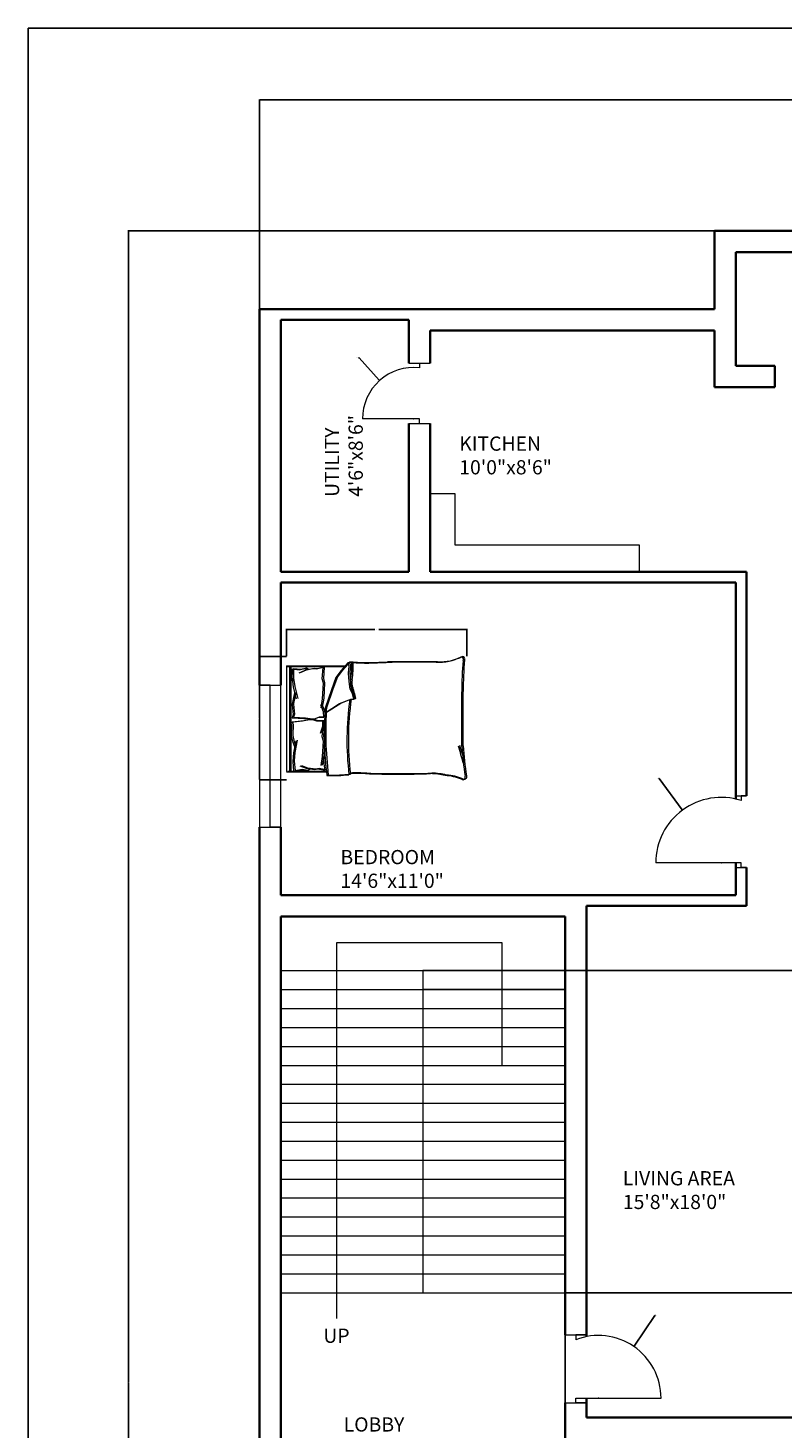
# Model space of a CAD drawing. Units: inches. Extents: x 1902 to 2626, y 1199 to 2408.
# Tile 6 of 9: x 1902 to 2220, y 1817 to 2408. Entities that reach past the tile are written whole.
import ezdxf

# ---------------------------------------------------------------- set-up
doc = ezdxf.new("R2010")
doc.units = ezdxf.units.IN
for name, color, linetype, lineweight in [('A-ANNO-DIMS', 2, 'Continuous', 18), ('A-ANNO-SYMB', 52, 'Continuous', 13), ('A-ANNO-TTLB', 7, 'Continuous', 25), ('A-AREA-IDEN', 7, 'Continuous', 18), ('A-DOOR', 31, 'Continuous', 18), ('A-FLOR-CASE', 8, 'Continuous', 18), ('A-FLOR-STRS', 52, 'Continuous', 18), ('A-FURN', 8, 'Continuous', 13), ('A-GLAZ', 181, 'Continuous', 18), ('A-WALL', 7, 'Continuous', 35)]:
    doc.layers.add(name, color=color, linetype=linetype, lineweight=lineweight)
doc.styles.get("Standard").update_dxf_attribs({"font": 'arial.ttf'})
doc.dimstyles.get("Standard").update_dxf_attribs({"dimtxt": 0.18, "dimasz": 0.18, "dimexe": 0.18, "dimexo": 0.0625, "dimgap": 0.09, "dimtad": 0, "dimtih": 1, "dimtoh": 1, "dimdec": 4, "dimzin": 0, "dimdsep": 46, "dimtxsty": 'Standard', "dimcen": 0.09, "dimadec": 0, "dimazin": 0, "dimtfac": 1, "dimtdec": 4, "dimtofl": 0, "dimtmove": 0, "dimatfit": 3, "dimfxl": 1, "dimtolj": 1, "dimtzin": 0, "dimarcsym": 0})

# ---------------------------------------------------------------- blocks, each defined once
blk = doc.blocks.new('BED-DOUBLE')
for p, q in [((-0.01, 48.09), (0.59, 48.09)), ((-0.01, 48.09), (-0.01, 3.46)), ((-0.01, 47.87), (24.84, 47.87)), ((-0.01, 47.87), (24.84, 47.87)), ((0.59, 48.09), (25.44, 48.09)), ((0.59, 48.09), (25.44, 48.09)), ((1.43, 3.25), (1.43, 47.87)), ((1.43, 3.25), (1.43, 47.87)), ((2.02, 3.46), (2.02, 48.09)), ((2.02, 3.46), (2.02, 48.09)), ((15.47, 47.34), (12.54, 46.62)), ((15.47, 47.34), (12.54, 46.62)), ((16.07, 47.56), (13.14, 46.83)), ((16.07, 47.56), (13.14, 46.83)), ((15.09, 42.55), (15.47, 47.34)), ((15.09, 42.55), (15.47, 47.34)), ((15.69, 42.77), (16.07, 47.56)), ((15.69, 42.77), (16.07, 47.56)), ((25.9, 49.37), (22.87, 45.91)), ((25.9, 49.37), (22.87, 45.91)), ((26.5, 49.58), (23.46, 46.12)), ((26.5, 49.58), (23.46, 46.12)), ((27.53, 49.44), (25.9, 49.37, 3.61)), ((27.53, 49.44), (25.9, 49.37, 3.61)), ((26.48, 47.93), (25.9, 49.37)), ((26.48, 47.93), (25.9, 49.37)), ((26.19, 45.04), (26.48, 47.93)), ((26.19, 45.04), (26.48, 47.93)), ((28.13, 49.66), (26.5, 49.58, 3.61)), ((28.13, 49.66), (26.5, 49.58, 3.61)), ((27.08, 48.15), (26.5, 49.58)), ((27.08, 48.15), (26.5, 49.58)), ((26.79, 45.26), (27.08, 48.15)), ((26.79, 45.25), (27.08, 48.15)), ((2.38, 46.8), (2.29, 41.75)), ((2.38, 46.8), (2.29, 41.75)), ((2.29, 41.75), (2.37, 42.69)), ((2.29, 41.75), (2.37, 42.69)), ((2.37, 42.69), (2.86, 39.14)), ((2.37, 42.69), (2.86, 39.14)), ((2.38, 46.8), (5.38, 46.44)), ((2.38, 46.8), (5.38, 46.44)), ((2.98, 47.01), (2.89, 41.97)), ((2.98, 47.01), (2.89, 41.96)), ((2.89, 41.97), (2.97, 42.9)), ((2.89, 41.96), (2.97, 42.9)), ((2.97, 42.9), (3.46, 39.36)), ((2.97, 42.9), (3.46, 39.35)), ((2.98, 47.01), (5.98, 46.66)), ((2.98, 47.01), (5.98, 46.66)), ((7.7, 46.05), (5.2, 44.94)), ((7.7, 46.05), (5.2, 44.94)), ((5.38, 46.44), (7.78, 47)), ((5.38, 46.44), (7.78, 47)), ((8.3, 46.26), (5.8, 45.16)), ((8.3, 46.26), (5.8, 45.16)), ((5.98, 46.66), (8.38, 47.21)), ((5.98, 46.66), (8.38, 47.21)), ((11.04, 46.8), (7.7, 46.05)), ((11.04, 46.8), (7.7, 46.05)), ((7.78, 47), (8.76, 46.52)), ((7.78, 47), (8.76, 46.52)), ((11.64, 47.01), (8.3, 46.26)), ((11.64, 47.01), (8.3, 46.26)), ((8.38, 47.21), (9.35, 46.73)), ((8.38, 47.21), (9.35, 46.73)), ((12.54, 46.62), (11.04, 46.8)), ((12.54, 46.62), (11.04, 46.8)), ((13.14, 46.83), (11.64, 47.01)), ((13.14, 46.83), (11.64, 47.01)), ((15.61, 40.72), (15.09, 42.55)), ((15.61, 40.72), (15.09, 42.55)), ((16.21, 40.93), (15.69, 42.77)), ((16.21, 40.93), (15.69, 42.77)), ((20.84, 43.16), (18.97, 37.96)), ((20.84, 43.16), (18.97, 37.96)), ((21.44, 43.38), (19.56, 38.17)), ((21.44, 43.38), (19.56, 38.17)), ((22.87, 45.91), (20.84, 43.16)), ((22.87, 45.91), (20.84, 43.16)), ((23.46, 46.12), (21.44, 43.38)), ((23.46, 46.12), (21.44, 43.38)), ((26.48, 41.43), (26.19, 45.04)), ((26.48, 41.43), (26.19, 45.04)), ((26.91, 38.25), (26.48, 41.43)), ((26.91, 38.24), (26.48, 41.43)), ((27.08, 41.64), (26.79, 45.26)), ((27.08, 41.64), (26.79, 45.25)), ((27.51, 38.46), (27.08, 41.64)), ((27.51, 38.46), (27.08, 41.64)), ((2.86, 39.14), (4.12, 34.08)), ((2.86, 39.14), (4.12, 34.08)), ((3.42, 36.61), (2.87, 34.68)), ((3.42, 36.61), (2.87, 34.68)), ((3.46, 39.36), (4.72, 34.29)), ((3.46, 39.35), (4.72, 34.29)), ((4.02, 36.82), (3.47, 34.89)), ((4.02, 36.82), (3.47, 34.89)), ((15.21, 34.18), (15.61, 40.72)), ((15.21, 34.18), (15.61, 40.72)), ((15.81, 34.39), (16.21, 40.93)), ((15.81, 34.39), (16.21, 40.93)), ((18.97, 37.96), (16.23, 30.17)), ((18.97, 37.96), (16.23, 30.17)), ((19.56, 38.17), (16.82, 30.38)), ((19.56, 38.17), (16.82, 30.38)), ((27.78, 36.37), (26.91, 38.25)), ((27.78, 36.36), (26.91, 38.24)), ((28.38, 36.58), (27.51, 38.46)), ((28.38, 36.58), (27.51, 38.46)), ((28.36, 34.05), (27.78, 36.37)), ((28.36, 34.05), (27.78, 36.36)), ((28.96, 34.26), (28.38, 36.58)), ((28.96, 34.26), (28.38, 36.58)), ((73.99, 14.07), (73.99, 37.05)), ((73.99, 14.07), (73.99, 37.05)), ((74.59, 14.28), (74.59, 37.27)), ((74.59, 14.28), (74.59, 37.27)), ((2.87, 34.68), (2.36, 31.94)), ((2.87, 34.68), (2.36, 31.94)), ((2.36, 31.94), (2.38, 31.64)), ((2.36, 31.94), (2.38, 31.64)), ((2.38, 31.64), (2.78, 27.51)), ((2.38, 31.64), (2.78, 27.51)), ((3.47, 34.89), (2.96, 32.16)), ((3.47, 34.89), (2.96, 32.16)), ((2.96, 32.16), (2.98, 31.86)), ((2.96, 32.16), (2.98, 31.86)), ((2.98, 31.86), (3.37, 27.72)), ((2.98, 31.86), (3.37, 27.72)), ((15.63, 28.72), (14.43, 31.58)), ((15.63, 28.72), (14.43, 31.58)), ((14.59, 30.41), (15.21, 34.18)), ((14.59, 30.41), (15.21, 34.18)), ((16.22, 28.93), (15.02, 31.8)), ((16.22, 28.93), (15.02, 31.8)), ((15.18, 30.62), (15.81, 34.39)), ((15.18, 30.62), (15.81, 34.39)), ((16.23, 28.26), (22.29, 32.17)), ((16.23, 28.26), (22.29, 32.17)), ((16.82, 28.47), (22.89, 32.38)), ((16.82, 28.47), (22.89, 32.38)), ((22.29, 32.17), (26.48, 33.76)), ((22.29, 32.17), (26.48, 33.76)), ((22.89, 32.38), (27.08, 33.98)), ((22.89, 32.38), (27.08, 33.98)), ((26.48, 33.76), (28.36, 34.05)), ((26.48, 33.76), (28.36, 34.05)), ((27.08, 33.98), (28.96, 34.26)), ((27.08, 33.98), (28.96, 34.26)), ((1.74, 24.27), (6.74, 24.81)), ((1.74, 24.27), (6.74, 24.81)), ((2.28, 22.92), (1.74, 24.27)), ((2.28, 22.92), (1.74, 24.27)), ((2.78, 27.51), (2.32, 26.13)), ((2.78, 27.51), (2.32, 26.13)), ((2.32, 26.13), (7.34, 25.9)), ((2.32, 26.13), (7.34, 25.9)), ((2.34, 24.48), (7.33, 25.02)), ((2.34, 24.48), (7.33, 25.02)), ((2.88, 23.13), (2.34, 24.48)), ((2.88, 23.13), (2.34, 24.48)), ((3.37, 27.72), (2.92, 26.34)), ((3.37, 27.72), (2.92, 26.34)), ((2.92, 26.34), (7.94, 26.11)), ((2.92, 26.34), (7.94, 26.11)), ((6.74, 24.81), (9.71, 25.35)), ((6.74, 24.81), (9.71, 25.35)), ((7.33, 25.02), (10.3, 25.56)), ((7.33, 25.02), (10.3, 25.56)), ((7.34, 25.9), (10.34, 25.55)), ((7.34, 25.9), (10.34, 25.55)), ((7.94, 26.11), (10.94, 25.76)), ((7.94, 26.11), (10.94, 25.76)), ((9.71, 25.35), (10.92, 25.35)), ((9.71, 25.35), (10.92, 25.35)), ((10.3, 25.56), (11.52, 25.56)), ((10.3, 25.56), (11.52, 25.56)), ((10.34, 25.55), (11.55, 25.62)), ((10.34, 25.55), (11.55, 25.62)), ((10.92, 25.35), (12.68, 24.81)), ((10.92, 25.35), (12.68, 24.81)), ((10.94, 25.76), (12.15, 25.84)), ((10.94, 25.76), (12.15, 25.84)), ((11.52, 25.56), (13.27, 25.02)), ((11.52, 25.56), (13.27, 25.02)), ((11.55, 25.62), (13.27, 26.27)), ((11.55, 25.62), (13.27, 26.27)), ((12.15, 25.84), (13.87, 26.48)), ((12.15, 25.84), (13.87, 26.48)), ((12.68, 24.81), (15.18, 24.81)), ((12.68, 24.81), (15.18, 24.81)), ((13.27, 26.27), (15.77, 26.43)), ((13.27, 26.27), (15.77, 26.43)), ((13.27, 25.02), (15.78, 25.02)), ((13.27, 25.02), (15.78, 25.02)), ((13.87, 26.48), (16.37, 26.64)), ((13.87, 26.48), (16.37, 26.64)), ((15.18, 24.81), (15.18, 22.51)), ((15.18, 24.81), (15.18, 22.51)), ((15.77, 26.43), (15.63, 28.72)), ((15.77, 26.43), (15.63, 28.72)), ((15.78, 25.02), (15.78, 22.72)), ((15.78, 25.02), (15.78, 22.72)), ((16.37, 26.64), (16.22, 28.93)), ((16.37, 26.64), (16.22, 28.93)), ((2.15, 18.76), (2.28, 22.92)), ((2.15, 18.76), (2.28, 22.92)), ((2.15, 18.46), (2.15, 18.76)), ((2.15, 18.46), (2.15, 18.76)), ((2.82, 15.76), (2.15, 18.46)), ((2.82, 15.76), (2.15, 18.46)), ((2.74, 18.98), (2.88, 23.13)), ((2.74, 18.98), (2.88, 23.13)), ((2.74, 18.68), (2.74, 18.98)), ((2.74, 18.68), (2.74, 18.98)), ((3.42, 15.98), (2.74, 18.68)), ((3.42, 15.98), (2.74, 18.68)), ((15.18, 22.51), (14.16, 19.57)), ((15.18, 22.51), (14.16, 19.57)), ((15.78, 22.72), (14.76, 19.79)), ((15.78, 22.72), (14.76, 19.79)), ((15.09, 18.1), (15.47, 22.9)), ((15.09, 18.1), (15.47, 22.9)), ((15.61, 16.27), (15.09, 18.1)), ((15.61, 16.27), (15.09, 18.1)), ((15.69, 18.32), (16.07, 23.11)), ((15.69, 18.32), (16.07, 23.11)), ((16.21, 16.49), (15.69, 18.32)), ((16.21, 16.49), (15.69, 18.32)), ((3.5, 13.88), (2.82, 15.76)), ((3.5, 13.87), (2.82, 15.76)), ((3.09, 11.31), (4.04, 16.44)), ((3.09, 11.31), (4.04, 16.44)), ((4.09, 14.09), (3.42, 15.98)), ((4.09, 14.09), (3.42, 15.98)), ((3.69, 11.52), (4.63, 16.65)), ((3.69, 11.52), (4.63, 16.65)), ((15.21, 9.73), (15.61, 16.27)), ((15.21, 9.73), (15.61, 16.27)), ((15.81, 9.94), (16.21, 16.49)), ((15.81, 9.94), (16.21, 16.49)), ((2.8, 7.64), (2.82, 7.74)), ((2.8, 7.64), (2.82, 7.74)), ((3.11, 3.64), (2.8, 7.64)), ((3.11, 3.64), (2.8, 7.64)), ((2.82, 7.74), (3.09, 11.31)), ((2.82, 7.74), (3.09, 11.31)), ((3.4, 7.86), (3.42, 7.95)), ((3.4, 7.86), (3.42, 7.95)), ((3.71, 3.86), (3.4, 7.86)), ((3.71, 3.86), (3.4, 7.86)), ((3.42, 7.95), (3.69, 11.52)), ((3.42, 7.95), (3.69, 11.52)), ((14.59, 5.96), (15.21, 9.73)), ((14.59, 5.96), (15.21, 9.73)), ((15.18, 6.18), (15.81, 9.94)), ((15.18, 6.18), (15.81, 9.94)), ((15.21, 9.73), (15.51, 8.67)), ((15.21, 9.73), (15.51, 8.67)), ((15.51, 8.67), (16.19, 3.91)), ((15.51, 8.67), (16.19, 3.91)), ((15.81, 9.94), (16.11, 8.88)), ((15.81, 9.94), (16.11, 8.88)), ((16.11, 8.88), (16.78, 4.12)), ((16.11, 8.88), (16.78, 4.12)), ((16.91, 3.25), (-0.01, 3.25)), ((16.91, 3.25), (-0.01, 3.25)), ((17.5, 3.46), (0.59, 3.46)), ((17.5, 3.46), (0.59, 3.46)), ((3.09, 3.64), (6.06, 4.18)), ((3.09, 3.64), (6.06, 4.18)), ((3.69, 3.85), (6.66, 4.39)), ((3.69, 3.85), (6.66, 4.39)), ((8.36, 4.72), (5.79, 5.67)), ((8.36, 4.72), (5.79, 5.67)), ((6.06, 4.18), (8.49, 3.78)), ((6.06, 4.18), (8.49, 3.78)), ((8.95, 4.93), (6.39, 5.88)), ((8.95, 4.93), (6.39, 5.88)), ((6.66, 4.39), (9.09, 3.99)), ((6.66, 4.39), (9.09, 3.99)), ((11.73, 4.18), (8.36, 4.72)), ((11.73, 4.18), (8.36, 4.72)), ((8.49, 3.78), (9.44, 4.32)), ((8.49, 3.78), (9.44, 4.32)), ((12.33, 4.39), (8.95, 4.93)), ((12.33, 4.39), (8.95, 4.93)), ((9.09, 3.99), (10.03, 4.53)), ((9.09, 3.99), (10.03, 4.53)), ((13.22, 4.45), (11.73, 4.18)), ((13.22, 4.45), (11.73, 4.18)), ((13.81, 4.66), (12.33, 4.39)), ((13.81, 4.66), (12.33, 4.39)), ((16.19, 3.91), (13.22, 4.45)), ((16.19, 3.91), (13.22, 4.45)), ((16.78, 4.12), (13.81, 4.66)), ((16.78, 4.12), (13.81, 4.66))]:
    blk.add_line(p, q)
for centre, radius, start, end in [((-6.22, 47.93), 33.79, 349.87628, 2.56571), ((-6.22, 47.93), 33.79, 349.87628, 2.56571), ((33.9, 170.19), 120.92, 266.97912, 273.83645), ((33.9, 170.19), 120.92, 266.97912, 273.83645), ((-5.62, 48.14), 33.79, 349.87628, 2.56571), ((-5.62, 48.14), 33.79, 349.87628, 2.56571), ((34.5, 170.41), 120.92, 266.97912, 273.83645), ((34.5, 170.41), 120.92, 266.97912, 273.83645), ((63.32, -4210.02), 4259.62, 90.00217, 90.28689), ((63.32, -4210.02), 4259.62, 90.00217, 90.28689), ((63.92, -4209.8), 4259.62, 90.00217, 90.28689), ((63.92, -4209.8), 4259.62, 90.00217, 90.28689), ((64.11, 71.12), 21.54, 267.47136, 296.46809), ((64.11, 71.12), 21.54, 267.47136, 296.46809), ((64.71, 71.33), 21.54, 267.47136, 296.46809), ((64.71, 71.33), 21.54, 267.47136, 296.46809), ((73.64, 50.81), 1.03, 332.65876, 86.02002), ((73.64, 50.81), 1.03, 332.65876, 86.02002), ((198.21, 38.43), 124.23, 174.4998, 180.63509), ((198.21, 38.43), 124.23, 174.4998, 180.63509), ((74.24, 51.02), 1.03, 332.65876, 86.02002), ((74.24, 51.02), 1.03, 332.65876, 86.02002), ((198.8, 38.64), 124.23, 174.4998, 180.63509), ((198.8, 38.64), 124.23, 174.4998, 180.63509), ((32.74, 40.85), 5.81, 168.6608, 203.73842), ((32.74, 40.85), 5.81, 168.6608, 203.73842), ((33.33, 41.06), 5.81, 168.6608, 203.73842), ((33.33, 41.06), 5.81, 168.6608, 203.73842), ((1.38, 29.09), 27.69, 10.66171, 19.88058), ((1.38, 29.09), 27.69, 10.66171, 19.88058), ((1.98, 29.31), 27.69, 10.66171, 19.88058), ((1.98, 29.31), 27.69, 10.66171, 19.88058), ((169.99, 19.95), 154.04, 176.08655, 186.78213), ((169.99, 19.95), 154.04, 176.08655, 186.78213), ((170.58, 20.16), 154.04, 176.08655, 186.78213), ((170.58, 20.16), 154.04, 176.08655, 186.78213), ((145.95, 16.58), 120.47, 171.78449, 186.90062), ((145.95, 16.58), 120.47, 171.78449, 186.90062), ((146.55, 16.8), 120.47, 171.78449, 186.90062), ((146.55, 16.8), 120.47, 171.78449, 186.90062), ((28.42, 34.21), 0.172, 250.24637, 1.13765), ((28.42, 34.21), 0.172, 250.24637, 1.13765), ((29.01, 34.43), 0.172, 250.24637, 1.13765), ((29.01, 34.43), 0.172, 250.24637, 1.13765), ((-22.15, -16.08), 99.41, 13.38322, 17.70533), ((-22.15, -16.08), 99.41, 13.38322, 17.70533), ((-21.55, -15.86), 99.41, 13.38322, 17.70533), ((-21.55, -15.86), 99.41, 13.38322, 17.70533), ((187.53, 20.01), 113.69, 182.99578, 189.40907), ((187.53, 20.01), 113.69, 182.99578, 189.40907), ((188.12, 20.22), 113.69, 182.99578, 189.40907), ((188.12, 20.22), 113.69, 182.99578, 189.40907), ((18.76, 79.52), 77.79, 268.72178, 275.60397), ((18.76, 79.52), 77.79, 268.72178, 275.60397), ((19.36, 79.74), 77.79, 268.72178, 275.60397), ((19.36, 79.74), 77.79, 268.72178, 275.60397), ((29.1, -156.22), 158.84, 88.4762, 91.00819), ((29.1, -156.22), 158.84, 88.4762, 91.00819), ((29.7, -156), 158.84, 88.4762, 91.00819), ((29.7, -156.01), 158.84, 88.4762, 91.00819), ((47.26, 452.71), 450.36, 268.22771, 271.71854), ((47.26, 452.71), 450.36, 268.22771, 271.71854), ((47.85, 452.92), 450.36, 268.22771, 271.71854), ((47.85, 452.92), 450.36, 268.22771, 271.71854), ((60.24, -25.11), 27.67, 76.06484, 88.91125), ((60.24, -25.11), 27.67, 76.06484, 88.91125), ((60.83, -24.9), 27.67, 76.06484, 88.91125), ((60.83, -24.9), 27.67, 76.06484, 88.91125), ((65.61, -20.22), 22, 67.97508, 86.652), ((65.61, -20.22), 22, 67.97508, 86.652), ((66.21, -20.01), 22, 67.97508, 86.652), ((66.21, -20.01), 22, 67.97508, 86.652), ((74.43, 1.02), 1.02, 236.17358, 23.47814), ((74.43, 1.02), 1.02, 236.17358, 23.47814), ((75.03, 1.23), 1.02, 236.17358, 23.47814), ((75.03, 1.23), 1.02, 236.17358, 23.47814)]:
    blk.add_arc(centre, radius, start, end)
blk = doc.blocks.new('WINDOW-60-A')
for p, q in [((0, 9), (0, 0)), ((60, 9), (0, 9)), ((60, 4.5), (60, 9)), ((60, 9), (60, 0)), ((0, 0), (0, 4.5)), ((0, 4.5), (60, 4.5)), ((0, 0), (60, 0))]:
    blk.add_line(p, q)
blk = doc.blocks.new('*D10')
at = {"layer": 'A-ANNO-DIMS', "color": 0, "lineweight": -2, "transparency": 16777216}
for p, q in [((2010.79, 2142.84), (2010.79, 2154.38)), ((2010.97, 2154.2), (2048.05, 2154.2)), ((2086.76, 2154.2), (2049.69, 2154.2)), ((2086.94, 2142.84), (2086.94, 2154.38))]:
    blk.add_line(p, q, dxfattribs=at)
at = {"layer": 'A-ANNO-DIMS', "color": 0, "transparency": 16777216}
for points in [[(2010.97, 2154.23), (2010.97, 2154.17), (2010.79, 2154.2)], [(2086.76, 2154.23), (2086.76, 2154.17), (2086.94, 2154.2)]]:
    blk.add_solid(points, dxfattribs=at)
at = {"layer": 'Defpoints', "color": 0, "transparency": 16777216}
for p in [(2086.94, 2154.2), (2010.79, 2142.78), (2086.94, 2142.78)]:
    blk.add_point(p, dxfattribs=at)
at = {"layer": 'A-ANNO-DIMS', "color": 0, "transparency": 16777216, "insert": (2048.87, 2154.2), "char_height": 0.18, "attachment_point": 5}
blk.add_mtext('\\A1;BED 76 TYP.', dxfattribs=at)
blk = doc.blocks.new('*D11')
at = {"layer": 'A-ANNO-DIMS', "color": 0, "lineweight": -2, "transparency": 16777216}
for p, q in [((2010.73, 2142.78), (1999.19, 2142.78)), ((1999.37, 2142.6), (1999.37, 2116.9)), ((1999.37, 2090.83), (1999.37, 2116.53)), ((2010.73, 2090.65), (1999.19, 2090.65))]:
    blk.add_line(p, q, dxfattribs=at)
at = {"layer": 'A-ANNO-DIMS', "color": 0, "transparency": 16777216}
for points in [[(1999.34, 2142.6), (1999.4, 2142.6), (1999.37, 2142.78)], [(1999.34, 2090.83), (1999.4, 2090.83), (1999.37, 2090.65)]]:
    blk.add_solid(points, dxfattribs=at)
at = {"layer": 'Defpoints', "color": 0, "transparency": 16777216}
for p in [(1999.37, 2142.78), (2010.79, 2142.78), (2010.79, 2090.65)]:
    blk.add_point(p, dxfattribs=at)
at = {"layer": 'A-ANNO-DIMS', "color": 0, "transparency": 16777216, "insert": (1999.37, 2116.72), "char_height": 0.18, "attachment_point": 5}
blk.add_mtext('\\A1;52 TYP.', dxfattribs=at)
blk = doc.blocks.new('*D28')
at = {"layer": 'A-ANNO-DIMS', "color": 0, "lineweight": -2, "transparency": 16777216}
for p, q in [((1999.35, 2289.54), (1999.35, 2377.95)), ((1999.53, 2377.77), (2268.21, 2377.77)), ((2537.67, 2377.77), (2269, 2377.77)), ((2537.85, 2289.54), (2537.85, 2377.95))]:
    blk.add_line(p, q, dxfattribs=at)
at = {"layer": 'A-ANNO-DIMS', "color": 0, "transparency": 16777216}
for points in [[(1999.53, 2377.8), (1999.53, 2377.74), (1999.35, 2377.77)], [(2537.67, 2377.8), (2537.67, 2377.74), (2537.85, 2377.77)]]:
    blk.add_solid(points, dxfattribs=at)
at = {"layer": 'Defpoints', "color": 0, "transparency": 16777216}
for p in [(2537.85, 2377.77), (1999.35, 2289.47), (2537.85, 2289.47)]:
    blk.add_point(p, dxfattribs=at)
at = {"layer": 'A-ANNO-DIMS', "color": 0, "transparency": 16777216, "insert": (2268.6, 2377.77), "char_height": 0.18, "attachment_point": 5}
blk.add_mtext('\\A1;538.5', dxfattribs=at)
blk = doc.blocks.new('*D29')
at = {"layer": 'A-ANNO-DIMS', "color": 0, "lineweight": -2, "transparency": 16777216}
for p, q in [((2191.29, 2322.47), (1943.87, 2322.47)), ((1944.05, 2322.29), (1944.05, 1836.38)), ((1944.05, 1350.11), (1944.05, 1836.02)), ((2202.79, 1349.93), (1943.87, 1349.93))]:
    blk.add_line(p, q, dxfattribs=at)
at = {"layer": 'A-ANNO-DIMS', "color": 0, "transparency": 16777216}
for points in [[(1944.02, 2322.29), (1944.08, 2322.29), (1944.05, 2322.47)], [(1944.02, 1350.11), (1944.08, 1350.11), (1944.05, 1349.93)]]:
    blk.add_solid(points, dxfattribs=at)
at = {"layer": 'Defpoints', "color": 0, "transparency": 16777216}
for p in [(1944.05, 2322.47), (2191.35, 2322.47), (2202.85, 1349.93)]:
    blk.add_point(p, dxfattribs=at)
at = {"layer": 'A-ANNO-DIMS', "color": 0, "transparency": 16777216, "insert": (1944.05, 1836.2), "char_height": 0.18, "attachment_point": 5}
blk.add_mtext('\\A1;972.5', dxfattribs=at)
blk = doc.blocks.new('*D38')
at = {"layer": 'A-ANNO-DIMS', "color": 0, "lineweight": -2, "transparency": 16777216}
for p, q in [((2008.35, 1874.05), (2008.35, 1198.67)), ((2128.35, 1874.05), (2128.35, 1198.67)), ((2008.53, 1198.85), (2068.07, 1198.85)), ((2128.17, 1198.85), (2068.63, 1198.85))]:
    blk.add_line(p, q, dxfattribs=at)
at = {"layer": 'A-ANNO-DIMS', "color": 0, "transparency": 16777216}
for points in [[(2008.53, 1198.88), (2008.53, 1198.82), (2008.35, 1198.85)], [(2128.17, 1198.88), (2128.17, 1198.82), (2128.35, 1198.85)]]:
    blk.add_solid(points, dxfattribs=at)
at = {"layer": 'Defpoints', "color": 0, "transparency": 16777216}
for p in [(2008.35, 1874.11), (2128.35, 1874.11), (2128.35, 1198.85)]:
    blk.add_point(p, dxfattribs=at)
at = {"layer": 'A-ANNO-DIMS', "color": 0, "transparency": 16777216, "insert": (2068.35, 1198.85), "char_height": 0.18, "attachment_point": 5}
blk.add_mtext('\\A1;120', dxfattribs=at)
blk = doc.blocks.new('*D39')
at = {"layer": 'A-ANNO-DIMS', "color": 0, "lineweight": -2, "transparency": 16777216}
for p, q in [((2128.41, 2010.11), (2593.33, 2010.11)), ((2593.15, 2009.93), (2593.15, 1942.29)), ((2593.15, 1874.29), (2593.15, 1941.93)), ((2128.41, 1874.11), (2593.33, 1874.11))]:
    blk.add_line(p, q, dxfattribs=at)
at = {"layer": 'A-ANNO-DIMS', "color": 0, "transparency": 16777216}
for points in [[(2593.12, 2009.93), (2593.18, 2009.93), (2593.15, 2010.11)], [(2593.12, 1874.29), (2593.18, 1874.29), (2593.15, 1874.11)]]:
    blk.add_solid(points, dxfattribs=at)
at = {"layer": 'Defpoints', "color": 0, "transparency": 16777216}
for p in [(2128.35, 2010.11), (2593.15, 2010.11), (2128.35, 1874.11)]:
    blk.add_point(p, dxfattribs=at)
at = {"layer": 'A-ANNO-DIMS', "color": 0, "transparency": 16777216, "insert": (2593.15, 1942.11), "char_height": 0.18, "attachment_point": 5}
blk.add_mtext('\\A1;136', dxfattribs=at)
blk = doc.blocks.new('*D50')
at = {"layer": 'A-ANNO-DIMS', "color": 0, "lineweight": -2, "transparency": 16777216}
for p, q in [((2167.93, 2091.29), (2168.11, 2091.29)), ((2168.11, 2091.29), (2177.81, 2078.05)), ((2194.17, 2055.59), (2194.35, 2055.59)), ((2194.26, 2055.5), (2194.26, 2055.68))]:
    blk.add_line(p, q, dxfattribs=at)
at = {"layer": 'A-ANNO-DIMS', "color": 0, "transparency": 16777216}
blk.add_solid([(2177.83, 2078.07), (2177.78, 2078.03), (2177.92, 2077.9)], dxfattribs=at)
at = {"layer": 'Defpoints', "color": 0, "transparency": 16777216}
for p in [(2177.92, 2077.9), (2194.26, 2055.59)]:
    blk.add_point(p, dxfattribs=at)
at = {"layer": 'A-ANNO-DIMS', "color": 0, "transparency": 16777216, "insert": (2167.38, 2091.29), "char_height": 0.18, "attachment_point": 5}
blk.add_mtext('\\A1;R27.657', dxfattribs=at)
blk = doc.blocks.new('*D52')
at = {"layer": 'A-ANNO-DIMS', "color": 0, "lineweight": -2, "transparency": 16777216}
for p, q in [((2166.29, 1864.52), (2157.45, 1851.59)), ((2166.47, 1864.52), (2166.29, 1864.52)), ((2142.35, 1829.63), (2142.53, 1829.63)), ((2142.44, 1829.54), (2142.44, 1829.72))]:
    blk.add_line(p, q, dxfattribs=at)
at = {"layer": 'A-ANNO-DIMS', "color": 0, "transparency": 16777216}
blk.add_solid([(2157.42, 1851.6), (2157.47, 1851.57), (2157.34, 1851.44)], dxfattribs=at)
at = {"layer": 'Defpoints', "color": 0, "transparency": 16777216}
for p in [(2157.34, 1851.44), (2142.44, 1829.63)]:
    blk.add_point(p, dxfattribs=at)
at = {"layer": 'A-ANNO-DIMS', "color": 0, "transparency": 16777216, "insert": (2167.02, 1864.52), "char_height": 0.18, "attachment_point": 5}
blk.add_mtext('\\A1;R26.414', dxfattribs=at)
blk = doc.blocks.new('*D54')
at = {"layer": 'A-ANNO-DIMS', "color": 0, "lineweight": -2, "transparency": 16777216}
for p, q in [((2041.2, 2268.92), (2041.38, 2268.92)), ((2041.38, 2268.92), (2049.93, 2259.39)), ((2064.4, 2243.14), (2064.58, 2243.14)), ((2064.49, 2243.05), (2064.49, 2243.23))]:
    blk.add_line(p, q, dxfattribs=at)
at = {"layer": 'A-ANNO-DIMS', "color": 0, "transparency": 16777216}
blk.add_solid([(2049.95, 2259.41), (2049.91, 2259.37), (2050.05, 2259.25)], dxfattribs=at)
at = {"layer": 'Defpoints', "color": 0, "transparency": 16777216}
for p in [(2050.05, 2259.25), (2064.49, 2243.14)]:
    blk.add_point(p, dxfattribs=at)
at = {"layer": 'A-ANNO-DIMS', "color": 0, "transparency": 16777216, "insert": (2040.66, 2268.92), "char_height": 0.18, "attachment_point": 5}
blk.add_mtext('\\A1;R21.636', dxfattribs=at)

msp = doc.modelspace()

# ---------------------------------------------------------------- linework, layer by layer
at = {"layer": 'A-ANNO-SYMB'}
for p, q in [((2032.059, 1863.1842), (2032.059, 2022.0098)), ((2032.059, 2022.0098), (2101.6557, 2022.0098)), ((2101.6557, 2022.0098), (2101.6557, 1970.11)), ((2101.6557, 1970.11), (2101.6557, 1970.11))]:
    msp.add_line(p, q, dxfattribs=at)
at = {"layer": 'A-ANNO-TTLB'}
msp.add_lwpolyline([(1901.6928, 2408.1473), (2626.1646, 2408.1473), (2626.1646, 1206.3103), (1901.6928, 1206.3103)], close=True, dxfattribs=at)
at = {"layer": 'A-DOOR'}
for p, q in [((2062.3507, 2266.6459), (2071.3507, 2266.6459)), ((2066.8507, 2266.6459), (2066.8507, 2264.6459)), ((2066.8507, 2243.1399), (2042.8507, 2243.1399)), ((2062.3507, 2241.1399), (2071.3507, 2241.1399)), ((2066.8507, 2241.1399), (2066.8507, 2243.1399)), ((2200.3507, 2083.9588), (2204.8507, 2083.9588)), ((2204.8507, 2083.9588), (2202.6007, 2083.9588)), ((2202.6007, 2083.9588), (2202.6007, 2081.9588)), ((2202.6007, 2055.5908), (2166.6007, 2055.5908)), ((2200.3507, 2053.5908), (2204.8507, 2053.5908)), ((2202.6007, 2053.5908), (2202.6007, 2055.5908)), ((2204.8507, 2053.5908), (2202.6007, 2053.5908)), ((2128.3507, 1856.2475), (2137.3507, 1856.2475)), ((2137.3507, 1856.2475), (2132.8507, 1856.2475)), ((2132.8507, 1856.2475), (2132.8507, 1854.2475)), ((2128.3507, 1827.6338), (2137.3507, 1827.6338)), ((2132.8507, 1827.6338), (2132.8507, 1829.6338)), ((2132.8507, 1829.6338), (2168.8507, 1829.6338)), ((2137.3507, 1827.6338), (2132.8507, 1827.6338))]:
    msp.add_line(p, q, dxfattribs=at)
for centre, radius, start, end in [((2064.4863, 2243.1399), 21.6356, 83.7259546, 180), ((2194.2573, 2055.5908), 27.6566, 72.4414808, 180), ((2142.4363, 1829.6338), 26.4144, 0, 111.2780943)]:
    msp.add_arc(centre, radius, start, end, dxfattribs=at)
at = {"layer": 'A-FLOR-CASE'}
for p, q in [((2071.3507, 2211.5459), (2081.7541, 2211.5459)), ((2081.7541, 2211.5459), (2081.7541, 2189.8841)), ((2081.7541, 2189.8841), (2159.6685, 2189.8841)), ((2159.6685, 2189.8841), (2159.6685, 2178.4733))]:
    msp.add_line(p, q, dxfattribs=at)
at = {"layer": 'A-FLOR-STRS'}
for p, q in [((2008.3507, 2010.11), (2128.3507, 2010.11)), ((2128.3507, 2010.11), (2068.3507, 2010.11)), ((2068.3507, 2010.11), (2068.3507, 1874.11)), ((2008.3507, 2002.11), (2128.3507, 2002.11)), ((2128.3507, 2002.11), (2068.3507, 2002.11)), ((2008.3507, 1994.11), (2128.3507, 1994.11)), ((2008.3507, 1986.11), (2128.3507, 1986.11)), ((2008.3507, 1978.11), (2128.3507, 1978.11)), ((2008.3507, 1970.11), (2128.3507, 1970.11)), ((2008.3507, 1962.11), (2128.3507, 1962.11)), ((2008.3507, 1954.11), (2128.3507, 1954.11)), ((2008.3507, 1946.11), (2128.3507, 1946.11)), ((2008.3507, 1938.11), (2128.3507, 1938.11)), ((2008.3507, 1930.11), (2128.3507, 1930.11)), ((2008.3507, 1922.11), (2128.3507, 1922.11)), ((2008.3507, 1914.11), (2128.3507, 1914.11)), ((2008.3507, 1906.11), (2128.3507, 1906.11)), ((2008.3507, 1898.11), (2128.3507, 1898.11)), ((2008.3507, 1890.11), (2128.3507, 1890.11)), ((2008.3507, 1882.11), (2128.3507, 1882.11)), ((2008.3507, 1874.11), (2128.3507, 1874.11))]:
    msp.add_line(p, q, dxfattribs=at)
at = {"layer": 'A-GLAZ'}
msp.add_line((1999.3507, 2070.6537), (2008.3507, 2070.6537), dxfattribs=at)
at = {"layer": 'A-WALL'}
for p, q in [((2341.3507, 2322.4733), (2191.3507, 2322.4733)), ((2191.3507, 2322.4733), (2191.3507, 2289.4733)), ((2200.3507, 2280.4733), (2200.3507, 2313.4733)), ((2200.3507, 2313.4733), (2332.3507, 2313.4733)), ((1999.3507, 2289.4733), (2191.3507, 2289.4733)), ((1999.3507, 2289.4733), (1999.3507, 2130.6537)), ((1999.3507, 2289.4733), (2003.8507, 2289.4733)), ((2008.3507, 2284.9733), (2008.3507, 2178.4733)), ((2008.3507, 2284.9733), (2062.3507, 2284.9733)), ((2062.3507, 2284.9733), (2062.3507, 2277.5087)), ((2062.3507, 2277.5087), (2062.3507, 2266.6459)), ((2071.3507, 2280.4733), (2191.3507, 2280.4733)), ((2071.3507, 2280.4733), (2071.3507, 2277.5087)), ((2071.3507, 2280.4733), (2071.3507, 2266.6459)), ((2071.3507, 2266.6459), (2071.3507, 2277.5087)), ((2191.3507, 2280.4733), (2191.3507, 2265.8979)), ((2200.3507, 2280.4733), (2200.3507, 2265.8979)), ((2200.3507, 2280.4733), (2200.3507, 2265.4733)), ((2191.3507, 2256.4733), (2191.3507, 2265.8979)), ((2200.3507, 2265.4733), (2216.8872, 2265.4733)), ((2216.8872, 2265.4733), (2216.8872, 2256.4733)), ((2200.3507, 2256.4733), (2191.3507, 2256.4733)), ((2200.3507, 2256.4733), (2216.8872, 2256.4733)), ((2062.3507, 2241.1399), (2062.3507, 2235.4733)), ((2071.3507, 2241.1399), (2071.3507, 2235.4733)), ((2071.3507, 2241.1399), (2071.3507, 2178.4733)), ((2062.3507, 2235.4733), (2062.3507, 2178.4733)), ((2008.3507, 2178.4733), (2062.3507, 2178.4733)), ((2062.3507, 2178.4733), (2008.3507, 2178.4733)), ((2071.3507, 2178.4733), (2200.3507, 2178.4733)), ((2071.3507, 2178.4733), (2204.8507, 2178.4733)), ((2204.8507, 2178.4733), (2071.3507, 2178.4733)), ((2204.8507, 2178.4733), (2204.8507, 2083.9588)), ((2008.3507, 2173.9733), (2200.3507, 2173.9733)), ((2008.3507, 2173.9733), (2008.3507, 2130.6537)), ((2200.3507, 2173.9733), (2200.3507, 2082.5677)), ((1999.3507, 2070.6537), (1999.3507, 1571.1752)), ((2008.3507, 2070.6537), (2008.3507, 2041.9733)), ((2008.3507, 2070.6537), (2008.3507, 2041.9733)), ((2200.3507, 2055.5908), (2200.3507, 2041.9733)), ((2204.8507, 2053.5908), (2204.8507, 2041.9733)), ((2200.3507, 2041.9733), (2008.3507, 2041.9733)), ((2204.8507, 2041.9733), (2204.8507, 2037.4733)), ((2137.3507, 1866.5214), (2137.3507, 2037.4733)), ((2137.3507, 2037.4733), (2149.0985, 2037.4733)), ((2200.3507, 2037.4733), (2149.0985, 2037.4733)), ((2200.3507, 2037.4733), (2204.8507, 2037.4733)), ((2008.3507, 2032.9733), (2128.3507, 2032.9733)), ((2128.3507, 2032.9733), (2008.3507, 2032.9733)), ((2008.3507, 2032.9733), (2008.3507, 1747.7028)), ((2128.3507, 2032.9733), (2128.3507, 1866.5214)), ((2128.3507, 1874.11), (2128.3507, 1856.2475)), ((2137.3507, 1866.5214), (2137.3507, 1855.554)), ((2128.3507, 1827.6338), (2128.3507, 1806.4133)), ((2137.3507, 1829.6338), (2137.3507, 1821.4733)), ((2128.3507, 1824.8108), (2128.3507, 1806.4133)), ((2331.8507, 1821.4733), (2137.3507, 1821.4733))]:
    msp.add_line(p, q, dxfattribs=at)

# ---------------------------------------------------------------- block references
at = {"layer": 'A-FURN'}
msp.add_blockref('BED-DOUBLE', (2010.8, 2090.73), dxfattribs=at)
at = {"layer": 'A-GLAZ', "rotation": 90}
msp.add_blockref('WINDOW-60-A', (2008.354, 2070.6577), dxfattribs=at)

# ---------------------------------------------------------------- texts
at = {"layer": 'A-ANNO-SYMB', "insert": (2026.33, 1858.9297), "char_height": 6, "attachment_point": 1}
msp.add_mtext_dynamic_manual_height_columns('UP', width=56.095377, gutter_width=12.5, heights=[0], dxfattribs=at)
at = {"layer": 'A-AREA-IDEN', "insert": (2026.9875, 2210.1582), "char_height": 6, "attachment_point": 1, "rotation": 90}
msp.add_mtext_dynamic_manual_height_columns('UTILITY\\P4\'6"x8\'6"', width=198.914698, gutter_width=12.5, heights=[0], dxfattribs=at)
at = {"layer": 'A-AREA-IDEN', "char_height": 6, "attachment_point": 1}
for s, width, insert in [('KITCHEN\\P10\'0"x8\'6"', 161.007103, (2083.6923, 2235.6525)), ('BEDROOM\\P14\'6"x11\'0"', 198.892825, (2033.5486, 2061.0485)), ('LIVING AREA\\P15\'8"x18\'0"', 233.276262, (2152.7369, 1925.4327)), ('LOBBY\\P9\'6"x10\'6"', 191.395477, (2034.9094, 1821.4733))]:
    msp.add_mtext_dynamic_manual_height_columns(s, width=width, gutter_width=12.5, heights=[0], dxfattribs=dict(at, insert=insert))

# ---------------------------------------------------------------- dimensions: what is measured, and where the dimension line sits
at = {"layer": 'A-ANNO-DIMS'}
for base, p1, p2, override, picture, middle in [((2537.8507, 2377.7733), (1999.3507, 2289.4733), (2537.8507, 2289.4733), {"dimdec": 1, "dimlfac": 1, "dimrnd": 0, "dimzin": 0, "dimdsep": 46, "dimlunit": 2}, '*D28', (2268.6007, 2377.7733)), ((2128.3507, 1198.8475), (2008.3507, 1874.11), (2128.3507, 1874.11), {"dimdec": 0, "dimlfac": 1, "dimrnd": 0, "dimzin": 0, "dimdsep": 46, "dimlunit": 2}, '*D38', (2068.3507, 1198.8475))]:
    dim = msp.add_linear_dim(base=base, p1=p1, p2=p2, dimstyle='Standard', override=override, dxfattribs=at)
    dim.commit()
    dim.dimension.update_dxf_attribs({"geometry": picture, "text_midpoint": middle})
for base, p1, p2, override, picture, middle in [((1944.0507, 2322.4733), (2202.8507, 1349.9322), (2191.3507, 2322.4733), {"dimdec": 1, "dimlfac": 1, "dimrnd": 0, "dimzin": 0, "dimdsep": 46, "dimlunit": 2}, '*D29', (1944.0507, 1836.2028)), ((2593.1507, 2010.11), (2128.3507, 1874.11), (2128.3507, 2010.11), {"dimdec": 0, "dimlfac": 1, "dimrnd": 0, "dimzin": 0, "dimdsep": 46, "dimlunit": 2}, '*D39', (2593.1507, 1942.11))]:
    dim = msp.add_linear_dim(base=base, p1=p1, p2=p2, angle=90, dimstyle='Standard', override=override, dxfattribs=at)
    dim.commit()
    dim.dimension.update_dxf_attribs({"geometry": picture, "text_midpoint": middle})
for center, mpoint, picture, middle in [((2064.4863, 2243.1399), (2050.0479, 2259.2531), '*D54', (2040.6552, 2268.921)), ((2194.2573, 2055.5908), (2177.9152, 2077.9027), '*D50', (2167.3802, 2091.2899)), ((2142.4363, 1829.6338), (2157.3448, 1851.4388), '*D52', (2167.0193, 1864.5217))]:
    dim = msp.add_radius_dim(center=center, mpoint=mpoint, dimstyle='Standard', override={"dimdec": 3, "dimlfac": 1, "dimrnd": 0, "dimzin": 0, "dimdsep": 46, "dimlunit": 2}, dxfattribs=at)
    dim.commit()
    dim.dimension.update_dxf_attribs({"geometry": picture, "text_midpoint": middle, "dimtype": 164})
dim = msp.add_linear_dim(base=(2086.9403, 2154.2016), p1=(2010.7946, 2142.7798), p2=(2086.9403, 2142.7798), text='BED <> TYP.', dimstyle='Standard', override={"dimdec": 0, "dimlfac": 1, "dimrnd": 0, "dimzin": 0, "dimdsep": 46, "dimlunit": 2}, dxfattribs=at)
dim.commit()
dim.dimension.update_dxf_attribs({"geometry": '*D10', "text_midpoint": (2048.8675, 2154.2016)})
dim = msp.add_linear_dim(base=(1999.3728, 2142.7798), p1=(2010.7946, 2090.6538), p2=(2010.7946, 2142.7798), angle=90, text='<> TYP.', dimstyle='Standard', override={"dimdec": 0, "dimlfac": 1, "dimrnd": 0, "dimzin": 0, "dimdsep": 46, "dimlunit": 2}, dxfattribs=at)
dim.commit()
dim.dimension.update_dxf_attribs({"geometry": '*D11', "text_midpoint": (1999.3728, 2116.7168)})

doc.saveas('drawing.dxf')
